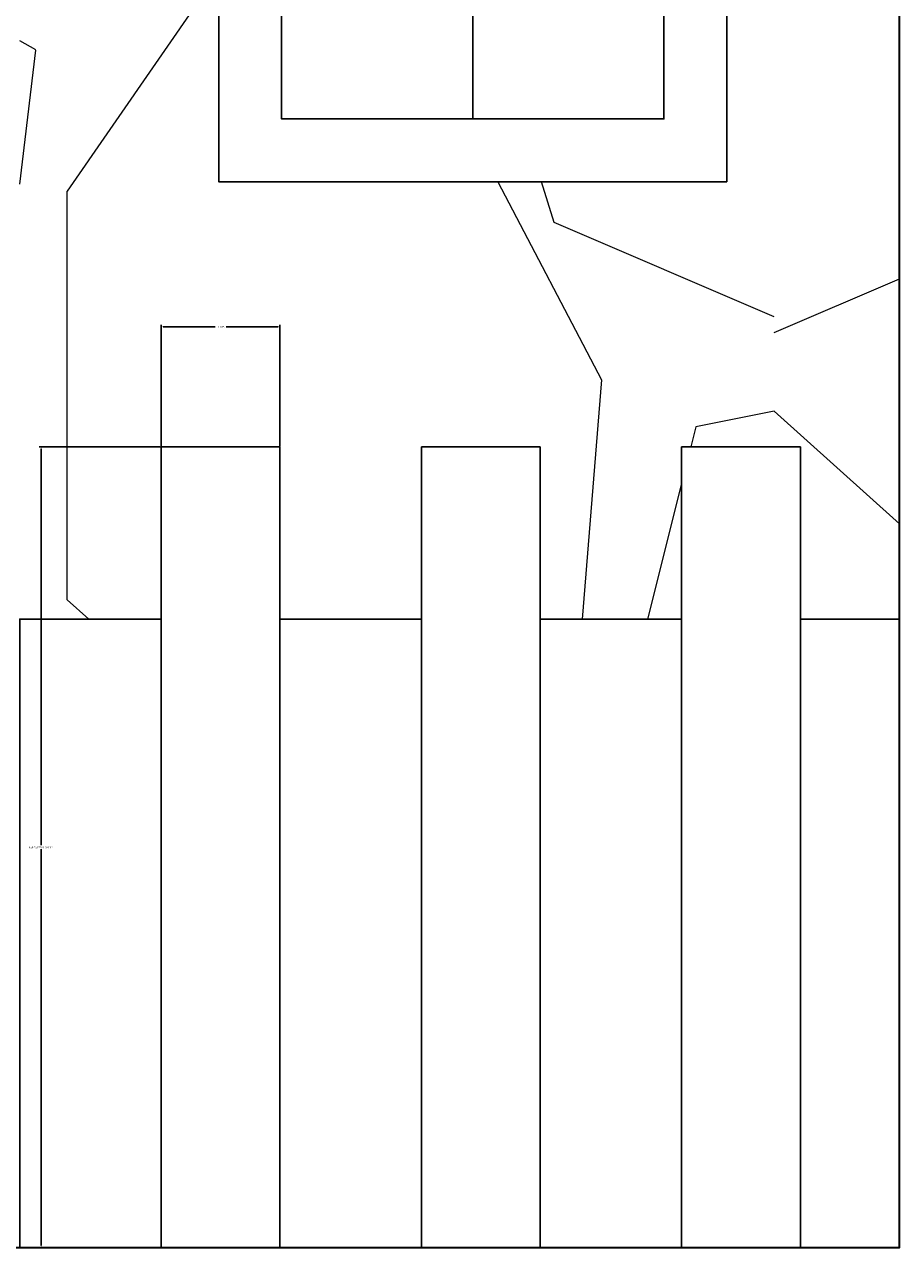
# Model space of a CAD drawing. Units: inches. Extents: x 3 to 303, y 4 to 326.
# Tile 3 of 6: x 220 to 303, y 4 to 120. Entities that reach past the tile are written whole.
import ezdxf

# ---------------------------------------------------------------- set-up
doc = ezdxf.new("R2010")
doc.units = ezdxf.units.IN
doc.header["$MEASUREMENT"] = 0
for name, color, linetype, lineweight in [('A-ANNO-DIMS', 2, 'Continuous', 18), ('A-ELEV', 7, 'Continuous', 35), ('A-ELEV-FENC', 8, 'Continuous', 25), ('A-ELEV-PATT', 8, 'Continuous', 13), ('A-GLAZ', 4, 'Continuous', 25)]:
    doc.layers.add(name, color=color, linetype=linetype, lineweight=lineweight)
doc.styles.get("Standard").update_dxf_attribs({"font": 'arial.ttf'})
doc.dimstyles.get("Standard").update_dxf_attribs({"dimtxt": 0.18, "dimasz": 0.18, "dimexe": 0.18, "dimexo": 0.0625, "dimgap": 0.09, "dimtad": 0, "dimtih": 1, "dimtoh": 1, "dimdec": 4, "dimzin": 0, "dimdsep": 46, "dimtxsty": 'Standard', "dimcen": 0.09, "dimadec": 0, "dimazin": 0, "dimtfac": 1, "dimtdec": 4, "dimtofl": 0, "dimtmove": 0, "dimatfit": 3, "dimfxl": 1, "dimtolj": 1, "dimtzin": 0, "dimarcsym": 0})

# ---------------------------------------------------------------- blocks, each defined once
blk = doc.blocks.new('FENCE-POST')
blk.add_lwpolyline([(-4.25465206888e-05, 76.44432969089668), (11.34032817950791, 76.44432969089668), (11.34032817950791, 0.0001748626421447), (-4.25465206888e-05, 0.0001748626421447)], close=True)
blk = doc.blocks.new('*D10')
at = {"layer": 'A-ANNO-DIMS', "color": 0, "lineweight": -2, "transparency": 16777216}
for p, q in [((232.6664574534794, 80.06132969089671), (221.0823342292413, 80.06132969089668)), ((221.2623342292413, 79.88132969089669), (221.2623342292414, 42.02238324539152)), ((221.2623342292414, 3.797174862642144), (221.2623342292414, 41.65612130814731)), ((232.6664574534794, 3.617174862642145), (221.0823342292413, 3.617174862642144))]:
    blk.add_line(p, q, dxfattribs=at)
at = {"layer": 'A-ANNO-DIMS', "color": 0, "transparency": 16777216}
for points in [[(221.2323342292414, 79.88132969089669), (221.2923342292413, 79.88132969089669), (221.2623342292413, 80.06132969089668)], [(221.2323342292414, 3.797174862642144), (221.2923342292413, 3.797174862642144), (221.2623342292414, 3.617174862642144)]]:
    blk.add_solid(points, dxfattribs=at)
at = {"layer": 'Defpoints', "color": 0, "transparency": 16777216}
for p in [(221.2623342292413, 80.06132969089668), (232.7289574534794, 80.06132969089671), (232.7289574534794, 3.617174862642145)]:
    blk.add_point(p, dxfattribs=at)
at = {"layer": 'A-ANNO-DIMS', "color": 0, "transparency": 16777216, "insert": (221.2623342292413, 41.83925227676935), "char_height": 0.18, "attachment_point": 5}
blk.add_mtext('\\A1;FENCE POST 76 TYP.', dxfattribs=at)
blk = doc.blocks.new('*D11')
at = {"layer": 'A-ANNO-DIMS', "color": 0, "lineweight": -2, "transparency": 16777216}
for p, q in [((232.7289574534793, 80.12382969089668), (232.7289574534793, 91.70795291513485)), ((232.9089574534793, 91.52795291513486), (237.8795248083081, 91.52795291513486)), ((243.8893281795079, 91.52795291513486), (238.9187608246792, 91.52795291513486)), ((244.0693281795079, 80.12382969089668), (244.0693281795079, 91.70795291513485))]:
    blk.add_line(p, q, dxfattribs=at)
at = {"layer": 'A-ANNO-DIMS', "color": 0, "transparency": 16777216}
for points in [[(232.9089574534793, 91.55795291513486), (232.9089574534793, 91.49795291513486), (232.7289574534793, 91.52795291513486)], [(243.8893281795079, 91.55795291513486), (243.8893281795079, 91.49795291513486), (244.0693281795079, 91.52795291513486)]]:
    blk.add_solid(points, dxfattribs=at)
at = {"layer": 'Defpoints', "color": 0, "transparency": 16777216}
for p in [(244.0693281795079, 91.52795291513486), (232.7289574534793, 80.06132969089668), (244.0693281795079, 80.06132969089668)]:
    blk.add_point(p, dxfattribs=at)
at = {"layer": 'A-ANNO-DIMS', "color": 0, "transparency": 16777216, "insert": (238.3991428164936, 91.52795291513486), "char_height": 0.18, "attachment_point": 5}
blk.add_mtext('\\A1;11 TYP.', dxfattribs=at)

msp = doc.modelspace()

# ---------------------------------------------------------------- hatches: boundary and pattern name
at = {"layer": 'A-ELEV-PATT'}
h = msp.add_hatch(dxfattribs=at)
h.set_pattern_fill('GRAVEL', color=256, scale=150, angle=90)
h.set_pattern_definition([(318.012787504, (-159.711805372533, 82.49771926165387), (1350, -1200.000000000009), [20.1804, -1997.863207061055]), (274.969740728, (-144.711805372533, 68.99771926165387), (-150.0000000000051, 1799.999999999996), [34.6302, -3428.388714184499]), (222.510447078, (-141.711805372533, 34.49771926165386), (1649.99999999998, 1500.000000000017), [24.4182, -2417.404889414955]), (357.273689006, (-104.211805372533, -24.00228073834614), (-3000.000000000003, 150.0000000000038), [31.5357, -3122.03370624435]), (22.83365417800003, (-72.71180537253304, -25.50228073834614), (-1800.000000000004, -749.9999999999982), [30.92325, -3061.405969213245]), (87.27368900599996, (-44.21180537253303, -13.50228073834614), (-150.000000000004, -3000.000000000003), [31.5357, -3122.03370624435]), (127.6942404667, (-42.71180537253303, 17.99771926165385), (1499.999999999996, -1950), [41.70435, -4128.7272823374]), (162.2553283749, (-68.21180537253304, 50.99771926165385), (-3300.000000000001, 1050.000000000004), [39.3732, -3897.948224522009]), (211.429565615, (-105.711805372533, 62.99771926165385), (-1949.999999999998, -1200.000000000003), [31.6425, -3132.610966459349]), (265.236358309, (-132.711805372533, 46.49771926165387), (150.0000000000058, 1649.999999999997), [36.1248, -1770.114386818845]), (312.397437798, (-135.711805372533, 10.49771926165386), (1649.999999999996, -1799.999999999994), [46.71719999999999, -4625.006250719235]), (228.814074834, (-102.711805372533, 124.4977192616538), (-900.0000000000001, -1050.000000000005), [15.94515, -1578.576721910205]), (261.4692343899999, (-113.211805372533, 112.4977192616538), (299.9999999999994, 1950), [30.33555, -3003.22671242355]), (315, (-117.711805372533, 82.49771926165386), (149.9999999999899, -2.58e-14), [21.21315, -190.918884355965]), (293.198590514, (-135.711805372533, 71.99771926165387), (-299.9999999999963, 749.9999999999984), [11.4237, -1130.942265879585]), (21.80140948600004, (-131.211805372533, 61.49771926165387), (-450.0000000000154, -149.9999999999525), [16.15545, -791.619271070175]), (120.9637565321, (-116.211805372533, 67.49771926165386), (-299.9999999999969, 450.0000000000079), [26.23935, -848.4034342267948]), (251.565051177, (-129.711805372533, 89.99771926165387), (149.9999999999965, 300.0000000000017), [18.97365, -455.3679990252599]), (106.389540334, (-131.211805372533, -25.50228073834614), (-450.0000000000064, 1499.999999999995), [26.57999999999999, -2631.42677200041]), (160.3461759419, (-138.711805372533, -0.0022807383461334), (1650.000000000509, -600.0000000001831), [22.29915, -2207.61116209785]), (23.19859051399996, (-159.711805372533, 89.99771926165387), (-749.9999999999986, -299.9999999999955), [22.84725, -1119.518715879585]), (73.61045966600004, (-138.711805372533, 98.99771926165387), (-450.0000000000066, -1499.999999999995), [26.58, -2631.42677200035]), (69.44395478000004, (-38.21180537253304, -25.50228073834615), (-300.0000000000037, -750.0000000000055), [25.632, -1255.968561797625]), (24.775140569, (-29.21180537253304, -1.502280738346144), (-1650, -750.0000000000007), [21.4767, -2126.196459491399]), (156.8014094864, (-9.711805372533028, 91.49771926165386), (-749.9999999999955, 299.9999999999972), [22.84725, -1119.518715879585]), (107.3540246363, (-30.71180537253303, 100.4977192616538), (599.9999999999943, -1949.999999999997), [25.14465, -2489.313542136001]), (159.4439547804, (-9.711805372533034, 17.99771926165385), (749.9999999999931, -300.0000000000011), [12.816, -1268.784561797625]), (191.309932474, (-9.711805372533028, 82.49771926165386), (-600.0000000000018, -149.9999999999945), [7.6485, -757.2044270389199]), (255.963756532, (-17.21180537253303, 80.99771926165386), (150.0000000000002, 449.9999999999937), [30.92325, -587.542593842655]), (276.009005957, (-24.71180537253303, 50.99771926165385), (-149.9999999999974, 1500.000000000007), [28.6575, -2837.088476181421]), (33.69006752600001, (-102.711805372533, 67.49771926165386), (-299.9999999999979, -149.999999999998), [21.6333, -519.1993913196]), (83.15722658699998, (-84.71180537253304, 79.49771926165386), (300.0000000000081, 2550.000000000002), [37.7691, -3739.134393604246]), (150.9453959009, (-80.21180537253302, 116.9977192616538), (1049.999999999996, -599.9999999999964), [15.4434, -1528.90112114805]), (180, (-93.71180537253304, 124.4977192616538), (-150, -150), [9, -141]), (210.256437164, (-29.21180537253303, 47.99771926165385), (1050.000000000001, 600.0000000000013), [20.8386, -2063.02799841747]), (138.0127875042, (-47.21180537253302, 37.49771926165386), (-1349.999999999996, 1200), [40.3608, -1977.682807061055]), (90, (-77.21180537253304, 64.49771926165386), (-150, 150), [39, -111]), (55.30484646900005, (-77.21180537253302, 103.4977192616538), (1049.999999999974, 1500.000000000021), [23.7171, -2347.9911451263]), (344.054604099, (-63.71180537253303, 122.9977192616538), (600.0000000000007, -150.0000000000057), [21.8403, -1070.176183392075]), (297.645975364, (-42.71180537253303, 116.9977192616538), (1500.000000000007, -2849.999999999993), [35.55975, -3520.42112733891]), (265.42607874, (-26.21180537253303, 85.49771926165386), (-150.0000000000003, -1949.999999999993), [37.61985, -3724.361011195335])])
h.paths.add_polyline_path([(303.2262632093826, 123.6171748626421), (303.2262632093826, 243.6171748626422), (303.2262632093826, 325.612924607852), (219.2262632093826, 325.612924607852), (219.2262632093826, 243.6171748626422), (219.2262632093826, 63.61717486264215), (232.7289574534793, 63.61717486264215), (232.7289574534793, 80.06132969089668), (244.0693281795079, 80.06132969089668), (244.0693281795079, 63.61717486264215), (257.5720224236046, 63.61717486264215), (257.5720224236046, 80.06132969089668), (268.9123931496332, 80.06132969089668), (268.9123931496332, 63.61717486264215), (282.4150873937299, 63.61717486264214), (282.4150873937299, 80.06132969089668), (293.7554581197585, 80.06132969089668), (293.7554581197585, 63.61717486264215), (303.2262632093826, 63.61717486264215)])
h.paths.add_polyline_path([(286.7238180358027, 105.3811659699868), (238.2183155441071, 105.3811659699868), (238.2183155441071, 300.6586406846385), (286.7238180358027, 300.6586406846385)], flags=16)
h.paths.add_polyline_path([(280.7238180358027, 111.3811659699868), (244.2183155441071, 111.3811659699868), (244.2183155441071, 294.6586406846385), (280.7238180358027, 294.6586406846385)], flags=0)

# ---------------------------------------------------------------- linework, layer by layer
at = {"layer": 'A-ELEV'}
for p, q in [((303.2262632093826, 3.617174862642144), (303.2262632093826, 123.6171748626421)), ((15.22626320938262, 3.617174862642137), (303.2262632093826, 3.617174862642144))]:
    msp.add_line(p, q, dxfattribs=at)
at = {"layer": 'A-ELEV-FENC'}
for points in [[(293.7554581197585, 63.61717486264215), (303.2262632093826, 63.61717486264215), (303.2262632093826, 3.617174862642144), (219.2262632093826, 3.617174862642144), (219.2262632093826, 63.61717486264215), (232.7289574534793, 63.61717486264215)], [(244.0693281795079, 63.61717486264215), (257.5720224236046, 63.61717486264215)], [(268.9123931496332, 63.61717486264215), (282.4150873937299, 63.61717486264215)]]:
    msp.add_lwpolyline(points, dxfattribs=at)
at = {"layer": 'A-GLAZ'}
msp.add_line((262.4710667899549, 294.6586406846385), (262.4710667899549, 111.3811659699868), dxfattribs=at)
for points in [[(238.2183155441071, 300.6586406846385), (286.7238180358027, 300.6586406846385), (286.7238180358027, 105.3811659699868), (238.2183155441071, 105.3811659699868)], [(244.2183155441071, 294.6586406846385), (280.7238180358027, 294.6586406846385), (280.7238180358027, 111.3811659699868), (244.2183155441071, 111.3811659699868)]]:
    msp.add_lwpolyline(points, close=True, dxfattribs=at)

# ---------------------------------------------------------------- block references
at = {"layer": 'A-ELEV-FENC'}
for p in [(232.729, 3.616999999999999), (257.5720649701253, 3.617000000000001), (282.4151299402506, 3.617000000000001)]:
    msp.add_blockref('FENCE-POST', p, dxfattribs=at)

# ---------------------------------------------------------------- dimensions: what is measured, and where the dimension line sits
at = {"layer": 'A-ANNO-DIMS'}
dim = msp.add_linear_dim(base=(244.0693281795079, 91.52795291513486), p1=(232.7289574534793, 80.06132969089668), p2=(244.0693281795079, 80.06132969089668), text='<> TYP.', dimstyle='Standard', override={"dimdec": 0, "dimlfac": 1, "dimrnd": 0, "dimzin": 0, "dimdsep": 46, "dimlunit": 2}, dxfattribs=at)
dim.commit()
dim.dimension.update_dxf_attribs({"geometry": '*D11', "text_midpoint": (238.3991428164936, 91.52795291513486)})
dim = msp.add_linear_dim(base=(221.2623342292413, 80.06132969089668), p1=(232.7289574534793, 3.617174862642143), p2=(232.7289574534793, 80.06132969089668), angle=90, text='FENCE POST <> TYP.', dimstyle='Standard', override={"dimdec": 0, "dimlfac": 1, "dimrnd": 0, "dimzin": 0, "dimdsep": 46, "dimlunit": 2}, dxfattribs=at)
dim.commit()
dim.dimension.update_dxf_attribs({"geometry": '*D10', "text_midpoint": (221.2623342292413, 41.83925227676935)})

doc.saveas('drawing.dxf')
